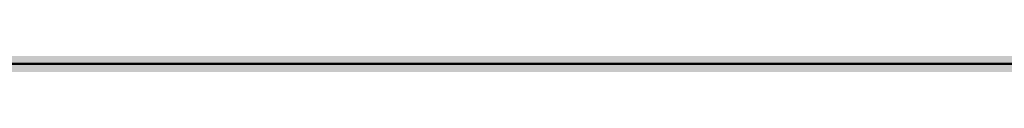
# Model space of a CAD drawing. Units: millimetres. Extents: x 0 to 2267, y 0 to 1823.
# Tile 89 of 256: x 1600.369 to 1605.705, y 1227.247 to 1227.247. Entities that reach past the tile are written whole.
import ezdxf

# ---------------------------------------------------------------- set-up
doc = ezdxf.new("R2010")
doc.units = ezdxf.units.MM
doc.header["$MEASUREMENT"] = 0
doc.layers.add('M-HATC', color=252, linetype='Continuous', lineweight=18)
doc.layers.add('M-OUTL', color=7, linetype='Continuous', lineweight=50)

msp = doc.modelspace()

# ---------------------------------------------------------------- hatches: boundary and pattern name
at = {"layer": 'M-HATC'}
h = msp.add_hatch(color=256, dxfattribs=at)
h.dxf.hatch_style = 1
h.paths.add_polyline_path([(2055.771, 1603.062), (1381.0868, 1603.062), (1381.0868, 1598.062), (2055.771, 1598.062)])
h.paths.add_polyline_path([(2055.771, 1598.062), (1381.0868, 1598.062), (1381.0868, 1593.062), (2055.771, 1593.062)])
h.paths.add_polyline_path([(2051.3074, 1536.7609), (1385.5504, 1536.7609), (1385.5504, 1526.7609), (1387.5504, 1526.7609), (1388.5366, 1525.0528), (1385.3319, 1521.2335), (1385.3319, 1521.2226), (2050.2542, 1522.7491), (2048.3212, 1525.0528), (2049.3074, 1526.7609), (2051.3074, 1526.7609)])
edge = h.paths.add_edge_path()
edge.add_arc((1847.5345, 1379.1492), 135, 222.603061, 222.890851, ccw=False)
edge.add_line((1748.1663, 1287.7656), (1683.0921, 1287.7656))
edge.add_arc((1583.7239, 1379.1492), 135, 317.109149, 317.396939, ccw=False)
edge.add_arc((1678.9686, 1290.6707), 5, 222.8909, 317.1091, ccw=False)
edge.add_arc((1774.2133, 1379.1492), 135, 222.603061, 222.890851, ccw=False)
edge.add_line((1674.8451, 1287.7656), (1609.7709, 1287.7656))
edge.add_arc((1510.4027, 1379.1492), 135, 317.109149, 317.396939, ccw=False)
edge.add_arc((1605.6474, 1290.6707), 5, 222.8909, 317.1091, ccw=False)
edge.add_arc((1700.8921, 1379.1492), 135, 222.603061, 222.890851, ccw=False)
edge.add_line((1601.5239, 1287.7656), (1536.4497, 1287.7656))
edge.add_arc((1437.0815, 1379.1492), 135, 317.109149, 317.396939, ccw=False)
edge.add_arc((1532.3262, 1290.6707), 5, 222.8909, 317.1091, ccw=False)
edge.add_arc((1627.5709, 1379.1492), 135, 222.603061, 222.890851, ccw=False)
edge.add_line((1528.2027, 1287.7656), (1505.9289, 1287.7656))
edge.add_spline(control_points=[(1505.9289, 1287.7656), (1504.2622, 1287.7656), (1504.2622, 1282.7656), (1505.9289, 1282.7656)], knot_values=[0, 0, 0, 0, 5, 5, 5, 5], degree=3, periodic=0)
edge.add_line((1505.9289, 1282.7656), (1930.9289, 1282.7656))
edge.add_spline(control_points=[(1930.9289, 1282.7656), (1932.5956, 1282.7656), (1932.5956, 1287.7656), (1930.9289, 1287.7656)], knot_values=[0, 0, 0, 0, 5, 5, 5, 5], degree=3, periodic=0)
edge.add_line((1930.9289, 1287.7656), (1903.0557, 1287.7656))
edge.add_arc((1803.6875, 1379.1492), 135, 317.109149, 317.396939, ccw=False)
edge.add_arc((1898.9322, 1290.6707), 5, 222.8909, 317.1091, ccw=False)
edge.add_arc((1994.1769, 1379.1492), 135, 222.603061, 222.890851, ccw=False)
edge.add_line((1894.8087, 1287.7656), (1829.7345, 1287.7656))
edge.add_arc((1730.3663, 1379.1492), 135, 317.109149, 317.396939, ccw=False)
edge.add_arc((1825.611, 1290.6707), 5, 222.8909, 317.1091, ccw=False)
edge.add_arc((1920.8557, 1379.1492), 135, 222.603061, 222.890851, ccw=False)
edge.add_line((1821.4875, 1287.7656), (1756.4133, 1287.7656))
edge.add_arc((1657.0451, 1379.1492), 135, 317.109149, 317.396939, ccw=False)
edge.add_arc((1752.2898, 1290.6707), 5, 222.8909, 317.1091, ccw=False)
edge = h.paths.add_edge_path()
edge.add_spline(control_points=[(1843.4289, 1227.2475), (1845.0956, 1227.2475), (1845.0956, 1232.2475), (1843.4289, 1232.2475)], knot_values=[0, 0, 0, 0, 5, 5, 5, 5], degree=3, periodic=0)
edge.add_line((1843.4289, 1232.2475), (1593.4289, 1232.2475))
edge.add_spline(control_points=[(1593.4289, 1232.2475), (1591.7622, 1232.2475), (1591.7622, 1227.2475), (1593.4289, 1227.2475)], knot_values=[0, 0, 0, 0, 5, 5, 5, 5], degree=3, periodic=0)
edge.add_line((1593.4289, 1227.2475), (1843.4289, 1227.2475))
h.paths.add_polyline_path([(1905.9289, 1127.4171), (1530.9289, 1127.4171, 0.414214), (1520.9289, 1117.4171), (1530.9289, 1117.4171), (1915.9289, 1117.4171, 0.414214)])
edge = h.paths.add_edge_path()
edge.add_arc((1397.0858, 1498.4078), 12.7299, 90.78215, 190.87871, ccw=False)
edge.add_line((1396.912, 1511.1365), (1428.0097, 1511.3488))
edge.add_line((1428.0097, 1511.3488), (1433.0097, 1511.3488))
edge.add_line((1433.0097, 1511.3488), (1434.439, 1511.3488))
edge.add_arc((1419.474, 1498.0804), 20, 41.561, 74.08211)
edge.add_line((1424.9592, 1517.3135), (1399.9351, 1517.2561))
edge.add_spline(control_points=[(1399.9307, 1517.2561), (1399.884, 1517.2131), (1399.8328, 1517.1689), (1399.7774, 1517.1236)], knot_values=[11.567499, 11.567499, 11.567499, 11.567499, 11.814249, 11.814249, 11.814249, 11.814249], degree=3, periodic=0)
edge.add_spline(control_points=[(1399.6328, 1517.0099), (1399.5831, 1516.9721), (1399.5307, 1516.9338), (1399.4759, 1516.8947)], knot_values=[11.167718, 11.167718, 11.167718, 11.167718, 11.365188, 11.365188, 11.365188, 11.365188], degree=3, periodic=0)
edge.add_spline(control_points=[(1399.3398, 1516.8001), (1399.1514, 1516.6719), (1398.9384, 1516.5377), (1398.704, 1516.3994)], knot_values=[10.376405, 10.376405, 10.376405, 10.376405, 11.00994, 11.00994, 11.00994, 11.00994], degree=3, periodic=0)
edge.add_spline(control_points=[(1398.6572, 1516.3719), (1398.5789, 1516.326), (1398.4983, 1516.2797), (1398.4155, 1516.2331)], knot_values=[10.125175, 10.125175, 10.125175, 10.125175, 10.334406, 10.334406, 10.334406, 10.334406], degree=3, periodic=0)
edge.add_spline(control_points=[(1398.2642, 1516.1487), (1398.196, 1516.1111), (1398.1263, 1516.0732), (1398.0555, 1516.0351)], knot_values=[9.832246, 9.832246, 9.832246, 9.832246, 9.999658, 9.999658, 9.999658, 9.999658], degree=3, periodic=0)
edge.add_spline(control_points=[(1397.9987, 1516.0048), (1397.7312, 1515.8621), (1397.446, 1515.7171), (1397.1466, 1515.5714)], knot_values=[9.161808, 9.161808, 9.161808, 9.161808, 9.787769, 9.787769, 9.787769, 9.787769], degree=3, periodic=0)
edge.add_spline(control_points=[(1397.1466, 1515.5714), (1396.8418, 1515.423), (1396.5222, 1515.274), (1396.1914, 1515.1262)], knot_values=[8.524455, 8.524455, 8.524455, 8.524455, 9.161808, 9.161808, 9.161808, 9.161808], degree=3, periodic=0)
edge.add_spline(control_points=[(1396.0777, 1515.0756), (1395.9854, 1515.0348), (1395.8922, 1514.994), (1395.7983, 1514.9534)], knot_values=[8.275193, 8.275193, 8.275193, 8.275193, 8.451726, 8.451726, 8.451726, 8.451726], degree=3, periodic=0)
edge.add_spline(control_points=[(1395.6018, 1514.8691), (1395.4997, 1514.8257), (1395.3968, 1514.7824), (1395.2932, 1514.7394)], knot_values=[7.962917, 7.962917, 7.962917, 7.962917, 8.152764, 8.152764, 8.152764, 8.152764], degree=3, periodic=0)
edge.add_spline(control_points=[(1395.2116, 1514.7057), (1394.8278, 1514.5475), (1394.4345, 1514.3929), (1394.0364, 1514.2442)], knot_values=[7.21254, 7.21254, 7.21254, 7.21254, 7.913148, 7.913148, 7.913148, 7.913148], degree=3, periodic=0)
edge.add_spline(control_points=[(1394.0364, 1514.2442), (1393.7076, 1514.1214), (1393.3754, 1514.0027), (1393.0427, 1513.8895)], knot_values=[6.633733, 6.633733, 6.633733, 6.633733, 7.21254, 7.21254, 7.21254, 7.21254], degree=3, periodic=0)
edge.add_spline(control_points=[(1392.8214, 1513.815), (1392.7198, 1513.7812), (1392.6181, 1513.7479), (1392.5166, 1513.7152)], knot_values=[6.328796, 6.328796, 6.328796, 6.328796, 6.505493, 6.505493, 6.505493, 6.505493], degree=3, periodic=0)
edge.add_spline(control_points=[(1392.5166, 1513.7152), (1392.3187, 1513.6515), (1392.1212, 1513.59), (1391.9244, 1513.531)], knot_values=[5.984605, 5.984605, 5.984605, 5.984605, 6.328796, 6.328796, 6.328796, 6.328796], degree=3, periodic=0)
edge.add_spline(control_points=[(1391.7915, 1513.4915), (1391.3122, 1513.3501), (1390.8384, 1513.2239), (1390.3784, 1513.1171)], knot_values=[5.066697, 5.066697, 5.066697, 5.066697, 5.907055, 5.907055, 5.907055, 5.907055], degree=3, periodic=0)
edge.add_spline(control_points=[(1390.3784, 1513.1171), (1390.1797, 1513.071), (1389.9836, 1513.0284), (1389.7907, 1512.9899)], knot_values=[4.70367, 4.70367, 4.70367, 4.70367, 5.066695, 5.066695, 5.066695, 5.066695], degree=3, periodic=0)
edge.add_spline(control_points=[(1389.422, 1512.9204), (1389.2459, 1512.8892), (1389.0729, 1512.8617), (1388.9036, 1512.8381)], knot_values=[4.130571, 4.130571, 4.130571, 4.130571, 4.469816, 4.469816, 4.469816, 4.469816], degree=3, periodic=0)
edge.add_spline(control_points=[(1388.9036, 1512.8381), (1388.591, 1512.7946), (1388.2911, 1512.7644), (1388.0071, 1512.7494)], knot_values=[3.504031, 3.504031, 3.504031, 3.504031, 4.130571, 4.130571, 4.130571, 4.130571], degree=3, periodic=0)
edge.add_spline(control_points=[(1387.9356, 1512.7459), (1387.8538, 1512.7423), (1387.7733, 1512.74), (1387.6944, 1512.739)], knot_values=[3.268866, 3.268866, 3.268866, 3.268866, 3.451164, 3.451164, 3.451164, 3.451164], degree=3, periodic=0)
edge.add_spline(control_points=[(1387.3351, 1512.7443), (1387.2076, 1512.7499), (1387.0847, 1512.7597), (1386.967, 1512.7739)], knot_values=[2.670686, 2.670686, 2.670686, 2.670686, 2.984, 2.984, 2.984, 2.984], degree=3, periodic=0)
edge.add_spline(control_points=[(1386.8327, 1512.7922), (1386.8209, 1512.7941), (1386.8092, 1512.7959), (1386.7975, 1512.7979)], knot_values=[2.516981, 2.516981, 2.516981, 2.516981, 2.549528, 2.549528, 2.549528, 2.549528], degree=3, periodic=0)
edge.add_spline(control_points=[(1386.4526, 1512.8735), (1386.4257, 1512.881), (1386.3993, 1512.889), (1386.3733, 1512.8972)], knot_values=[2.095869, 2.095869, 2.095869, 2.095869, 2.17941, 2.17941, 2.17941, 2.17941], degree=3, periodic=0)
edge.add_spline(control_points=[(1386.0691, 1513.0189), (1386.0634, 1513.0217), (1386.0577, 1513.0246), (1386.052, 1513.0275)], knot_values=[1.72453, 1.72453, 1.72453, 1.72453, 1.745933, 1.745933, 1.745933, 1.745933], degree=3, periodic=0)
edge.add_arc((1399.474, 1498.0804), 20, 131.82432, 180)
edge.add_arc((1630.3336, 1505.5484), 250.9708, 181.705176, 236.427975)
edge.add_arc((1605.3399, 1483.3044), 218.7822, 238.660829, 243.34961)
edge.add_arc((1647.0911, 1510.3592), 262.8986, 183.129836, 237.853442, ccw=False)
h.paths.add_polyline_path([(1406.5369, 1391.9644, 0.149382), (1491.5506, 1296.4418, -0.129517)], flags=17)
edge = h.paths.add_edge_path()
edge.add_arc((2037.3838, 1498.0804), 20, 0, 48.26587)
edge.add_spline(control_points=[(2050.6973, 1513.0052), (2050.6512, 1512.9847), (2050.6034, 1512.9655), (2050.5539, 1512.9477)], knot_values=[1.835652, 1.835652, 1.835652, 1.835652, 2.000781, 2.000781, 2.000781, 2.000781], degree=3, periodic=0)
edge.add_spline(control_points=[(2050.4616, 1512.9166), (2050.479, 1512.9221), (2050.4963, 1512.9277), (2050.5133, 1512.9335)], knot_values=[2.045477, 2.045477, 2.045477, 2.045477, 2.101389, 2.101389, 2.101389, 2.101389], degree=3, periodic=0)
edge.add_spline(control_points=[(2050.129, 1512.8342), (2050.1984, 1512.8473), (2050.2657, 1512.8623), (2050.3308, 1512.8792)], knot_values=[2.237629, 2.237629, 2.237629, 2.237629, 2.435841, 2.435841, 2.435841, 2.435841], degree=3, periodic=0)
edge.add_spline(control_points=[(2050.0946, 1512.8278), (2050.1061, 1512.8299), (2050.1176, 1512.832), (2050.129, 1512.8342)], knot_values=[2.435841, 2.435841, 2.435841, 2.435841, 2.468321, 2.468321, 2.468321, 2.468321], degree=3, periodic=0)
edge.add_spline(control_points=[(2049.7843, 1512.7851), (2049.8552, 1512.7922), (2049.9243, 1512.8008), (2049.9917, 1512.8109)], knot_values=[2.563852, 2.563852, 2.563852, 2.563852, 2.748541, 2.748541, 2.748541, 2.748541], degree=3, periodic=0)
edge.add_spline(control_points=[(2049.4052, 1512.7617), (2049.5364, 1512.7653), (2049.6629, 1512.773), (2049.7843, 1512.7851)], knot_values=[2.748541, 2.748541, 2.748541, 2.748541, 3.064882, 3.064882, 3.064882, 3.064882], degree=3, periodic=0)
edge.add_spline(control_points=[(2049.1698, 1512.7597), (2049.2336, 1512.7591), (2049.2965, 1512.7594), (2049.3584, 1512.7606)], knot_values=[3.102309, 3.102309, 3.102309, 3.102309, 3.2503, 3.2503, 3.2503, 3.2503], degree=3, periodic=0)
edge.add_spline(control_points=[(2048.8573, 1512.7691), (2048.9638, 1512.7638), (2049.068, 1512.7606), (2049.1698, 1512.7597)], knot_values=[3.2503, 3.2503, 3.2503, 3.2503, 3.486069, 3.486069, 3.486069, 3.486069], degree=3, periodic=0)
edge.add_spline(control_points=[(2048.6924, 1512.7789), (2048.3729, 1512.8009), (2048.0345, 1512.8411), (2047.6817, 1512.897)], knot_values=[3.606429, 3.606429, 3.606429, 3.606429, 4.2989, 4.2989, 4.2989, 4.2989], degree=3, periodic=0)
edge.add_spline(control_points=[(2047.6817, 1512.897), (2047.5458, 1512.9185), (2047.4077, 1512.9424), (2047.2678, 1512.9685)], knot_values=[4.2989, 4.2989, 4.2989, 4.2989, 4.565769, 4.565769, 4.565769, 4.565769], degree=3, periodic=0)
edge.add_spline(control_points=[(2047.2678, 1512.9685), (2047.1449, 1512.9914), (2047.0207, 1513.016), (2046.8951, 1513.0422)], knot_values=[4.565769, 4.565769, 4.565769, 4.565769, 4.799971, 4.799971, 4.799971, 4.799971], degree=3, periodic=0)
edge.add_spline(control_points=[(2046.8951, 1513.0422), (2046.5286, 1513.1188), (2046.1513, 1513.209), (2045.7676, 1513.3107)], knot_values=[4.799971, 4.799971, 4.799971, 4.799971, 5.483718, 5.483718, 5.483718, 5.483718], degree=3, periodic=0)
edge.add_spline(control_points=[(2045.7676, 1513.3107), (2045.3724, 1513.4154), (2044.9704, 1513.5322), (2044.5662, 1513.6588)], knot_values=[5.483718, 5.483718, 5.483718, 5.483718, 6.187866, 6.187866, 6.187866, 6.187866], degree=3, periodic=0)
edge.add_spline(control_points=[(2044.5662, 1513.6588), (2044.4149, 1513.7061), (2044.2633, 1513.7549), (2044.1116, 1513.8048)], knot_values=[6.187866, 6.187866, 6.187866, 6.187866, 6.451551, 6.451551, 6.451551, 6.451551], degree=3, periodic=0)
edge.add_spline(control_points=[(2044.1116, 1513.8048), (2043.9967, 1513.8427), (2043.8817, 1513.8813), (2043.7668, 1513.9205)], knot_values=[6.451551, 6.451551, 6.451551, 6.451551, 6.651434, 6.651434, 6.651434, 6.651434], degree=3, periodic=0)
edge.add_spline(control_points=[(2043.7668, 1513.9205), (2043.3716, 1514.0554), (2042.9774, 1514.1979), (2042.5886, 1514.3458)], knot_values=[6.651434, 6.651434, 6.651434, 6.651434, 7.338879, 7.338879, 7.338879, 7.338879], degree=3, periodic=0)
edge.add_spline(control_points=[(2042.5886, 1514.3458), (2042.1643, 1514.5071), (2041.7465, 1514.6749), (2041.3409, 1514.846)], knot_values=[7.338879, 7.338879, 7.338879, 7.338879, 8.089209, 8.089209, 8.089209, 8.089209], degree=3, periodic=0)
edge.add_spline(control_points=[(2041.3409, 1514.846), (2041.1028, 1514.9465), (2040.869, 1515.0481), (2040.6405, 1515.1502)], knot_values=[8.089209, 8.089209, 8.089209, 8.089209, 8.529587, 8.529587, 8.529587, 8.529587], degree=3, periodic=0)
edge.add_spline(control_points=[(2040.51, 1515.2089), (2040.0824, 1515.4022), (2039.6747, 1515.5971), (2039.295, 1515.7894)], knot_values=[8.613818, 8.613818, 8.613818, 8.613818, 9.44571, 9.44571, 9.44571, 9.44571], degree=3, periodic=0)
edge.add_spline(control_points=[(2039.295, 1515.7894), (2039.0618, 1515.9075), (2038.8391, 1516.0246), (2038.6288, 1516.1398)], knot_values=[9.44571, 9.44571, 9.44571, 9.44571, 9.956404, 9.956404, 9.956404, 9.956404], degree=3, periodic=0)
edge.add_spline(control_points=[(2038.6288, 1516.1398), (2038.5187, 1516.2001), (2038.4121, 1516.2598), (2038.309, 1516.3189)], knot_values=[9.956404, 9.956404, 9.956404, 9.956404, 10.223542, 10.223542, 10.223542, 10.223542], degree=3, periodic=0)
edge.add_spline(control_points=[(2038.309, 1516.3189), (2038.2138, 1516.3735), (2038.1216, 1516.4276), (2038.0328, 1516.481)], knot_values=[10.223542, 10.223542, 10.223542, 10.223542, 10.47051, 10.47051, 10.47051, 10.47051], degree=3, periodic=0)
edge.add_spline(control_points=[(2038.0328, 1516.481), (2037.7855, 1516.6296), (2037.5639, 1516.773), (2037.3722, 1516.909)], knot_values=[10.47051, 10.47051, 10.47051, 10.47051, 11.15767, 11.15767, 11.15767, 11.15767], degree=3, periodic=0)
edge.add_spline(control_points=[(2037.3722, 1516.909), (2037.2789, 1516.9752), (2037.1927, 1517.0396), (2037.1142, 1517.102)], knot_values=[11.15767, 11.15767, 11.15767, 11.15767, 11.49227, 11.49227, 11.49227, 11.49227], degree=3, periodic=0)
edge.add_spline(control_points=[(2036.8564, 1517.3259), (2036.9148, 1517.2692), (2036.9814, 1517.2103), (2037.0557, 1517.1492)], knot_values=[11.577341, 11.577341, 11.577341, 11.577341, 11.91035, 11.91035, 11.91035, 11.91035], degree=3, periodic=0)
edge.add_spline(control_points=[(2036.8074, 1517.3748), (2036.823, 1517.3587), (2036.8393, 1517.3424), (2036.8564, 1517.3259)], knot_values=[11.91035, 11.91035, 11.91035, 11.91035, 12.007402, 12.007402, 12.007402, 12.007402], degree=3, periodic=0)
edge.add_spline(control_points=[(2036.7017, 1517.494), (2036.7104, 1517.483), (2036.7196, 1517.4719), (2036.7291, 1517.4606)], knot_values=[12.184155, 12.184155, 12.184155, 12.184155, 12.255409, 12.255409, 12.255409, 12.255409], degree=3, periodic=0)
edge.add_spline(control_points=[(2036.6159, 1517.6205), (2036.62, 1517.613), (2036.6243, 1517.6055), (2036.6289, 1517.5979)], knot_values=[12.487913, 12.487913, 12.487913, 12.487913, 12.541035, 12.541035, 12.541035, 12.541035], degree=3, periodic=0)
edge.add_spline(control_points=[(2036.5635, 1517.786), (2036.5637, 1517.7794), (2036.5642, 1517.7726), (2036.565, 1517.7658)], knot_values=[12.911761, 12.911761, 12.911761, 12.911761, 12.968286, 12.968286, 12.968286, 12.968286], degree=3, periodic=0)
edge.add_spline(control_points=[(2036.6166, 1517.9304), (2036.6125, 1517.9259), (2036.6086, 1517.9212), (2036.6049, 1517.9165)], knot_values=[13.382527, 13.382527, 13.382527, 13.382527, 13.433791, 13.433791, 13.433791, 13.433791], degree=3, periodic=0)
edge.add_spline(control_points=[(2036.749, 1518.017), (2036.7361, 1518.0116), (2036.7239, 1518.006), (2036.7124, 1518.0002)], knot_values=[13.726299, 13.726299, 13.726299, 13.726299, 13.809928, 13.809928, 13.809928, 13.809928], degree=3, periodic=0)
edge.add_spline(control_points=[(2036.8604, 1518.0528), (2036.8386, 1518.0474), (2036.8181, 1518.0416), (2036.7988, 1518.0353)], knot_values=[13.910887, 13.910887, 13.910887, 13.910887, 14.02153, 14.02153, 14.02153, 14.02153], degree=3, periodic=0)
edge.add_line((2036.9639, 1518.0804), (2032.3838, 1518.0804))
edge.add_line((2032.3838, 1518.0804), (2027.3838, 1518.0804))
edge.add_line((2027.3838, 1518.0804), (2022.3838, 1518.0804))
edge.add_line((2022.3838, 1518.0804), (2017.3838, 1518.0804))
edge.add_arc((2017.3838, 1498.0804), 20, 90, 138.439)
edge.add_line((2002.4188, 1511.3488), (2003.8481, 1511.3488))
edge.add_line((2003.8481, 1511.3488), (2008.8481, 1511.3488))
edge.add_line((2008.8481, 1511.3488), (2039.772, 1511.1377))
edge.add_arc((2039.772, 1498.4078), 12.7299, -10.87871, 90, ccw=False)
edge.add_arc((1789.7668, 1510.3592), 262.8986, 302.146558, 356.870164, ccw=False)
edge.add_arc((1831.5179, 1483.3044), 218.7822, 296.65039, 301.339171)
edge.add_arc((1806.5242, 1505.5484), 250.9708, 303.572025, 358.294824)
h.paths.add_polyline_path([(2030.321, 1391.9644, -0.129517), (1945.3072, 1296.4418, 0.149382)], flags=17)
edge = h.paths.add_edge_path()
edge.add_spline(control_points=[(2037.2464, 1518.0821), (2037.2898, 1518.081), (2037.3355, 1518.0804), (2037.3838, 1518.0804)], knot_values=[0.000012, 0.000012, 0.000012, 0.000012, 0.144754, 0.144754, 0.144754, 0.144754], degree=3, periodic=0)
edge.add_line((2037.3357, 1518.0804), (2037.0096, 1518.0804))
edge.add_spline(control_points=[(2037.0096, 1518.0804), (2036.9822, 1518.0768), (2036.956, 1518.0727), (2036.9312, 1518.0681)], knot_values=[14.13465, 14.13465, 14.13465, 14.13465, 14.247197, 14.247197, 14.247197, 14.247197], degree=3, periodic=0)
edge.add_spline(control_points=[(2036.9312, 1518.0681), (2036.9276, 1518.0674), (2036.9241, 1518.0667), (2036.9205, 1518.0661)], knot_values=[14.118315, 14.118315, 14.118315, 14.118315, 14.13465, 14.13465, 14.13465, 14.13465], degree=3, periodic=0)
edge.add_spline(control_points=[(2036.9205, 1518.0661), (2036.9118, 1518.0644), (2036.9032, 1518.0626), (2036.8948, 1518.0608)], knot_values=[14.078086, 14.078086, 14.078086, 14.078086, 14.118315, 14.118315, 14.118315, 14.118315], degree=3, periodic=0)
edge.add_spline(control_points=[(2036.8948, 1518.0608), (2036.883, 1518.0583), (2036.8716, 1518.0556), (2036.8604, 1518.0528)], knot_values=[14.02153, 14.02153, 14.02153, 14.02153, 14.078086, 14.078086, 14.078086, 14.078086], degree=3, periodic=0)
edge.add_spline(control_points=[(2036.8604, 1518.0528), (2036.8386, 1518.0474), (2036.8181, 1518.0416), (2036.7988, 1518.0353)], knot_values=[13.910887, 13.910887, 13.910887, 13.910887, 14.02153, 14.02153, 14.02153, 14.02153], degree=3, periodic=0)
edge.add_spline(control_points=[(2036.7988, 1518.0353), (2036.7981, 1518.035), (2036.7974, 1518.0348), (2036.7967, 1518.0346)], knot_values=[13.906906, 13.906906, 13.906906, 13.906906, 13.910887, 13.910887, 13.910887, 13.910887], degree=3, periodic=0)
edge.add_spline(control_points=[(2036.7967, 1518.0346), (2036.7882, 1518.0318), (2036.7799, 1518.0289), (2036.7719, 1518.0259)], knot_values=[13.857826, 13.857826, 13.857826, 13.857826, 13.906906, 13.906906, 13.906906, 13.906906], degree=3, periodic=0)
edge.add_spline(control_points=[(2036.7719, 1518.0259), (2036.764, 1518.023), (2036.7564, 1518.02), (2036.749, 1518.017)], knot_values=[13.809928, 13.809928, 13.809928, 13.809928, 13.857826, 13.857826, 13.857826, 13.857826], degree=3, periodic=0)
edge.add_spline(control_points=[(2036.749, 1518.017), (2036.7361, 1518.0116), (2036.7239, 1518.006), (2036.7124, 1518.0002)], knot_values=[13.726299, 13.726299, 13.726299, 13.726299, 13.809928, 13.809928, 13.809928, 13.809928], degree=3, periodic=0)
edge.add_spline(control_points=[(2036.7124, 1518.0002), (2036.7121, 1518), (2036.7118, 1517.9999), (2036.7115, 1517.9997)], knot_values=[13.723993, 13.723993, 13.723993, 13.723993, 13.726299, 13.726299, 13.726299, 13.726299], degree=3, periodic=0)
edge.add_spline(control_points=[(2036.7115, 1517.9997), (2036.7063, 1517.9971), (2036.7013, 1517.9944), (2036.6965, 1517.9917)], knot_values=[13.686536, 13.686536, 13.686536, 13.686536, 13.723993, 13.723993, 13.723993, 13.723993], degree=3, periodic=0)
edge.add_spline(control_points=[(2036.6965, 1517.9917), (2036.6919, 1517.9891), (2036.6874, 1517.9865), (2036.6831, 1517.9839)], knot_values=[13.651251, 13.651251, 13.651251, 13.651251, 13.686536, 13.686536, 13.686536, 13.686536], degree=3, periodic=0)
edge.add_spline(control_points=[(2036.6831, 1517.9839), (2036.6764, 1517.9798), (2036.67, 1517.9757), (2036.6639, 1517.9714)], knot_values=[13.596804, 13.596804, 13.596804, 13.596804, 13.651251, 13.651251, 13.651251, 13.651251], degree=3, periodic=0)
edge.add_spline(control_points=[(2036.6639, 1517.9714), (2036.6636, 1517.9712), (2036.6633, 1517.9709), (2036.6629, 1517.9707)], knot_values=[13.593956, 13.593956, 13.593956, 13.593956, 13.596804, 13.596804, 13.596804, 13.596804], degree=3, periodic=0)
edge.add_spline(control_points=[(2036.6629, 1517.9707), (2036.6603, 1517.9689), (2036.6577, 1517.967), (2036.6552, 1517.9651)], knot_values=[13.570322, 13.570322, 13.570322, 13.570322, 13.593956, 13.593956, 13.593956, 13.593956], degree=3, periodic=0)
edge.add_spline(control_points=[(2036.6552, 1517.9651), (2036.6525, 1517.9631), (2036.6499, 1517.9611), (2036.6474, 1517.9591)], knot_values=[13.545477, 13.545477, 13.545477, 13.545477, 13.570322, 13.570322, 13.570322, 13.570322], degree=3, periodic=0)
edge.add_spline(control_points=[(2036.6474, 1517.9591), (2036.6472, 1517.9589), (2036.6471, 1517.9588), (2036.6469, 1517.9587)], knot_values=[13.543931, 13.543931, 13.543931, 13.543931, 13.545477, 13.545477, 13.545477, 13.545477], degree=3, periodic=0)
edge.add_spline(control_points=[(2036.6469, 1517.9587), (2036.6412, 1517.9541), (2036.6358, 1517.9494), (2036.6307, 1517.9447)], knot_values=[13.488237, 13.488237, 13.488237, 13.488237, 13.543931, 13.543931, 13.543931, 13.543931], degree=3, periodic=0)
edge.add_spline(control_points=[(2036.6307, 1517.9447), (2036.6282, 1517.9423), (2036.6257, 1517.9399), (2036.6233, 1517.9374)], knot_values=[13.460307, 13.460307, 13.460307, 13.460307, 13.488237, 13.488237, 13.488237, 13.488237], degree=3, periodic=0)
edge.add_spline(control_points=[(2036.6233, 1517.9374), (2036.6215, 1517.9356), (2036.6198, 1517.9338), (2036.6181, 1517.932)], knot_values=[13.439712, 13.439712, 13.439712, 13.439712, 13.460307, 13.460307, 13.460307, 13.460307], degree=3, periodic=0)
edge.add_spline(control_points=[(2036.6181, 1517.932), (2036.6176, 1517.9315), (2036.6171, 1517.9309), (2036.6166, 1517.9304)], knot_values=[13.433791, 13.433791, 13.433791, 13.433791, 13.439712, 13.439712, 13.439712, 13.439712], degree=3, periodic=0)
edge.add_spline(control_points=[(2036.6166, 1517.9304), (2036.6125, 1517.9259), (2036.6086, 1517.9212), (2036.6049, 1517.9165)], knot_values=[13.382527, 13.382527, 13.382527, 13.382527, 13.433791, 13.433791, 13.433791, 13.433791], degree=3, periodic=0)
edge.add_spline(control_points=[(2036.6049, 1517.9165), (2036.6026, 1517.9135), (2036.6004, 1517.9104), (2036.5982, 1517.9074)], knot_values=[13.350017, 13.350017, 13.350017, 13.350017, 13.382527, 13.382527, 13.382527, 13.382527], degree=3, periodic=0)
edge.add_spline(control_points=[(2036.5982, 1517.9074), (2036.5972, 1517.9059), (2036.5962, 1517.9043), (2036.5952, 1517.9028)], knot_values=[13.333922, 13.333922, 13.333922, 13.333922, 13.350017, 13.350017, 13.350017, 13.350017], degree=3, periodic=0)
edge.add_spline(control_points=[(2036.5952, 1517.9028), (2036.5945, 1517.9018), (2036.5939, 1517.9009), (2036.5933, 1517.8999)], knot_values=[13.323828, 13.323828, 13.323828, 13.323828, 13.333922, 13.333922, 13.333922, 13.333922], degree=3, periodic=0)
edge.add_spline(control_points=[(2036.5933, 1517.8999), (2036.5905, 1517.8955), (2036.5879, 1517.8909), (2036.5855, 1517.8864)], knot_values=[13.277545, 13.277545, 13.277545, 13.277545, 13.323828, 13.323828, 13.323828, 13.323828], degree=3, periodic=0)
edge.add_spline(control_points=[(2036.5855, 1517.8864), (2036.5836, 1517.8827), (2036.5817, 1517.8789), (2036.5801, 1517.8751)], knot_values=[13.240119, 13.240119, 13.240119, 13.240119, 13.277545, 13.277545, 13.277545, 13.277545], degree=3, periodic=0)
edge.add_spline(control_points=[(2036.5801, 1517.8751), (2036.5795, 1517.8739), (2036.579, 1517.8727), (2036.5785, 1517.8715)], knot_values=[13.228211, 13.228211, 13.228211, 13.228211, 13.240119, 13.240119, 13.240119, 13.240119], degree=3, periodic=0)
edge.add_spline(control_points=[(2036.5785, 1517.8715), (2036.578, 1517.8702), (2036.5774, 1517.869), (2036.5769, 1517.8677)], knot_values=[13.215717, 13.215717, 13.215717, 13.215717, 13.228211, 13.228211, 13.228211, 13.228211], degree=3, periodic=0)
edge.add_spline(control_points=[(2036.5769, 1517.8677), (2036.5755, 1517.864), (2036.5741, 1517.8603), (2036.5729, 1517.8565)], knot_values=[13.179847, 13.179847, 13.179847, 13.179847, 13.215717, 13.215717, 13.215717, 13.215717], degree=3, periodic=0)
edge.add_spline(control_points=[(2036.5729, 1517.8565), (2036.5713, 1517.8515), (2036.5699, 1517.8464), (2036.5687, 1517.8413)], knot_values=[13.132017, 13.132017, 13.132017, 13.132017, 13.179847, 13.179847, 13.179847, 13.179847], degree=3, periodic=0)
edge.add_spline(control_points=[(2036.5687, 1517.8413), (2036.5684, 1517.8402), (2036.5682, 1517.8392), (2036.568, 1517.8382)], knot_values=[13.122482, 13.122482, 13.122482, 13.122482, 13.132017, 13.132017, 13.132017, 13.132017], degree=3, periodic=0)
edge.add_spline(control_points=[(2036.568, 1517.8382), (2036.5676, 1517.8363), (2036.5672, 1517.8345), (2036.5669, 1517.8327)], knot_values=[13.105592, 13.105592, 13.105592, 13.105592, 13.122482, 13.122482, 13.122482, 13.122482], degree=3, periodic=0)
edge.add_spline(control_points=[(2036.5669, 1517.8327), (2036.5662, 1517.8292), (2036.5657, 1517.8257), (2036.5652, 1517.8222)], knot_values=[13.074063, 13.074063, 13.074063, 13.074063, 13.105592, 13.105592, 13.105592, 13.105592], degree=3, periodic=0)
edge.add_spline(control_points=[(2036.5652, 1517.8222), (2036.5652, 1517.8222), (2036.5652, 1517.8222), (2036.5652, 1517.8222)], knot_values=[13.074043, 13.074043, 13.074043, 13.074043, 13.074063, 13.074063, 13.074063, 13.074063], degree=3, periodic=0)
edge.add_spline(control_points=[(2036.5652, 1517.8222), (2036.5644, 1517.8164), (2036.5639, 1517.8106), (2036.5636, 1517.8046)], knot_values=[13.021884, 13.021884, 13.021884, 13.021884, 13.074043, 13.074043, 13.074043, 13.074043], degree=3, periodic=0)
edge.add_spline(control_points=[(2036.5636, 1517.8046), (2036.5636, 1517.804), (2036.5636, 1517.8034), (2036.5635, 1517.8028)], knot_values=[13.01674, 13.01674, 13.01674, 13.01674, 13.021884, 13.021884, 13.021884, 13.021884], degree=3, periodic=0)
edge.add_spline(control_points=[(2036.5635, 1517.8028), (2036.5634, 1517.8005), (2036.5634, 1517.7982), (2036.5634, 1517.7958)], knot_values=[12.996438, 12.996438, 12.996438, 12.996438, 13.01674, 13.01674, 13.01674, 13.01674], degree=3, periodic=0)
edge.add_spline(control_points=[(2036.5634, 1517.7958), (2036.5633, 1517.7926), (2036.5634, 1517.7893), (2036.5635, 1517.786)], knot_values=[12.968286, 12.968286, 12.968286, 12.968286, 12.996438, 12.996438, 12.996438, 12.996438], degree=3, periodic=0)
edge.add_spline(control_points=[(2036.5635, 1517.786), (2036.5637, 1517.7794), (2036.5642, 1517.7726), (2036.565, 1517.7658)], knot_values=[12.911761, 12.911761, 12.911761, 12.911761, 12.968286, 12.968286, 12.968286, 12.968286], degree=3, periodic=0)
edge.add_spline(control_points=[(2036.565, 1517.7658), (2036.565, 1517.7657), (2036.565, 1517.7656), (2036.565, 1517.7656)], knot_values=[12.911017, 12.911017, 12.911017, 12.911017, 12.911761, 12.911761, 12.911761, 12.911761], degree=3, periodic=0)
edge.add_spline(control_points=[(2036.565, 1517.7656), (2036.5654, 1517.7625), (2036.5658, 1517.7593), (2036.5663, 1517.7562)], knot_values=[12.88528, 12.88528, 12.88528, 12.88528, 12.911017, 12.911017, 12.911017, 12.911017], degree=3, periodic=0)
edge.add_spline(control_points=[(2036.5663, 1517.7562), (2036.5667, 1517.7534), (2036.5672, 1517.7506), (2036.5677, 1517.7478)], knot_values=[12.862519, 12.862519, 12.862519, 12.862519, 12.88528, 12.88528, 12.88528, 12.88528], degree=3, periodic=0)
edge.add_spline(control_points=[(2036.5677, 1517.7478), (2036.5678, 1517.7474), (2036.5679, 1517.7469), (2036.568, 1517.7465)], knot_values=[12.858885, 12.858885, 12.858885, 12.858885, 12.862519, 12.862519, 12.862519, 12.862519], degree=3, periodic=0)
edge.add_spline(control_points=[(2036.568, 1517.7465), (2036.5692, 1517.7399), (2036.5707, 1517.7332), (2036.5724, 1517.7264)], knot_values=[12.8053, 12.8053, 12.8053, 12.8053, 12.858885, 12.858885, 12.858885, 12.858885], degree=3, periodic=0)
edge.add_spline(control_points=[(2036.5724, 1517.7264), (2036.5734, 1517.7226), (2036.5745, 1517.7187), (2036.5756, 1517.7149)], knot_values=[12.775176, 12.775176, 12.775176, 12.775176, 12.8053, 12.8053, 12.8053, 12.8053], degree=3, periodic=0)
edge.add_spline(control_points=[(2036.5756, 1517.7149), (2036.5763, 1517.7125), (2036.577, 1517.7102), (2036.5778, 1517.7078)], knot_values=[12.756759, 12.756759, 12.756759, 12.756759, 12.775176, 12.775176, 12.775176, 12.775176], degree=3, periodic=0)
edge.add_spline(control_points=[(2036.5778, 1517.7078), (2036.5781, 1517.7067), (2036.5784, 1517.7057), (2036.5787, 1517.7047)], knot_values=[12.748742, 12.748742, 12.748742, 12.748742, 12.756759, 12.756759, 12.756759, 12.756759], degree=3, periodic=0)
edge.add_spline(control_points=[(2036.5787, 1517.7047), (2036.5808, 1517.6983), (2036.5831, 1517.6919), (2036.5856, 1517.6854)], knot_values=[12.69959, 12.69959, 12.69959, 12.69959, 12.748742, 12.748742, 12.748742, 12.748742], degree=3, periodic=0)
edge.add_spline(control_points=[(2036.5856, 1517.6854), (2036.5876, 1517.68), (2036.5898, 1517.6746), (2036.5921, 1517.6692)], knot_values=[12.659038, 12.659038, 12.659038, 12.659038, 12.69959, 12.69959, 12.69959, 12.69959], degree=3, periodic=0)
edge.add_spline(control_points=[(2036.5921, 1517.6692), (2036.594, 1517.6648), (2036.5959, 1517.6605), (2036.5979, 1517.6561)], knot_values=[12.626806, 12.626806, 12.626806, 12.626806, 12.659038, 12.659038, 12.659038, 12.659038], degree=3, periodic=0)
edge.add_spline(control_points=[(2036.5979, 1517.6561), (2036.5984, 1517.6551), (2036.5989, 1517.6541), (2036.5993, 1517.6531)], knot_values=[12.619394, 12.619394, 12.619394, 12.619394, 12.626806, 12.626806, 12.626806, 12.626806], degree=3, periodic=0)
edge.add_spline(control_points=[(2036.5993, 1517.6531), (2036.6043, 1517.6424), (2036.6099, 1517.6315), (2036.6159, 1517.6205)], knot_values=[12.541039, 12.541039, 12.541039, 12.541039, 12.619394, 12.619394, 12.619394, 12.619394], degree=3, periodic=0)
edge.add_spline(control_points=[(2036.6159, 1517.6205), (2036.6159, 1517.6205), (2036.6159, 1517.6205), (2036.6159, 1517.6205)], knot_values=[12.541035, 12.541035, 12.541035, 12.541035, 12.541039, 12.541039, 12.541039, 12.541039], degree=3, periodic=0)
edge.add_spline(control_points=[(2036.6159, 1517.6205), (2036.62, 1517.613), (2036.6243, 1517.6055), (2036.6289, 1517.5979)], knot_values=[12.487913, 12.487913, 12.487913, 12.487913, 12.541035, 12.541035, 12.541035, 12.541035], degree=3, periodic=0)
edge.add_spline(control_points=[(2036.6289, 1517.5979), (2036.6326, 1517.5916), (2036.6365, 1517.5853), (2036.6406, 1517.5789)], knot_values=[12.443982, 12.443982, 12.443982, 12.443982, 12.487913, 12.487913, 12.487913, 12.487913], degree=3, periodic=0)
edge.add_spline(control_points=[(2036.6406, 1517.5789), (2036.6414, 1517.5776), (2036.6423, 1517.5763), (2036.6431, 1517.5749)], knot_values=[12.434996, 12.434996, 12.434996, 12.434996, 12.443982, 12.443982, 12.443982, 12.443982], degree=3, periodic=0)
edge.add_spline(control_points=[(2036.6431, 1517.5749), (2036.6531, 1517.5596), (2036.6639, 1517.5439), (2036.6756, 1517.528)], knot_values=[12.329647, 12.329647, 12.329647, 12.329647, 12.434996, 12.434996, 12.434996, 12.434996], degree=3, periodic=0)
edge.add_spline(control_points=[(2036.6756, 1517.528), (2036.6839, 1517.5168), (2036.6925, 1517.5055), (2036.7017, 1517.494)], knot_values=[12.255409, 12.255409, 12.255409, 12.255409, 12.329647, 12.329647, 12.329647, 12.329647], degree=3, periodic=0)
edge.add_spline(control_points=[(2036.7017, 1517.494), (2036.7104, 1517.483), (2036.7196, 1517.4719), (2036.7291, 1517.4606)], knot_values=[12.184155, 12.184155, 12.184155, 12.184155, 12.255409, 12.255409, 12.255409, 12.255409], degree=3, periodic=0)
edge.add_spline(control_points=[(2036.7291, 1517.4606), (2036.7436, 1517.4435), (2036.759, 1517.4262), (2036.7753, 1517.4085)], knot_values=[12.075961, 12.075961, 12.075961, 12.075961, 12.184155, 12.184155, 12.184155, 12.184155], degree=3, periodic=0)
edge.add_spline(control_points=[(2036.7753, 1517.4085), (2036.7763, 1517.4075), (2036.7773, 1517.4064), (2036.7783, 1517.4054)], knot_values=[12.069502, 12.069502, 12.069502, 12.069502, 12.075961, 12.075961, 12.075961, 12.075961], degree=3, periodic=0)
edge.add_spline(control_points=[(2036.7783, 1517.4054), (2036.7877, 1517.3953), (2036.7974, 1517.385), (2036.8074, 1517.3748)], knot_values=[12.007402, 12.007402, 12.007402, 12.007402, 12.069502, 12.069502, 12.069502, 12.069502], degree=3, periodic=0)
edge.add_spline(control_points=[(2036.8074, 1517.3748), (2036.823, 1517.3587), (2036.8393, 1517.3424), (2036.8564, 1517.3259)], knot_values=[11.91035, 11.91035, 11.91035, 11.91035, 12.007402, 12.007402, 12.007402, 12.007402], degree=3, periodic=0)
edge.add_spline(control_points=[(2036.8564, 1517.3259), (2036.9148, 1517.2692), (2036.9814, 1517.2103), (2037.0557, 1517.1492)], knot_values=[11.577341, 11.577341, 11.577341, 11.577341, 11.91035, 11.91035, 11.91035, 11.91035], degree=3, periodic=0)
edge.add_spline(control_points=[(2037.0557, 1517.1492), (2037.0747, 1517.1336), (2037.0942, 1517.1179), (2037.1142, 1517.102)], knot_values=[11.49227, 11.49227, 11.49227, 11.49227, 11.577341, 11.577341, 11.577341, 11.577341], degree=3, periodic=0)
edge.add_spline(control_points=[(2037.1142, 1517.102), (2037.1927, 1517.0396), (2037.2789, 1516.9752), (2037.3722, 1516.909)], knot_values=[11.15767, 11.15767, 11.15767, 11.15767, 11.49227, 11.49227, 11.49227, 11.49227], degree=3, periodic=0)
edge.add_spline(control_points=[(2037.3722, 1516.909), (2037.5639, 1516.773), (2037.7855, 1516.6296), (2038.0328, 1516.481)], knot_values=[10.47051, 10.47051, 10.47051, 10.47051, 11.15767, 11.15767, 11.15767, 11.15767], degree=3, periodic=0)
edge.add_spline(control_points=[(2038.0328, 1516.481), (2038.1216, 1516.4276), (2038.2138, 1516.3735), (2038.309, 1516.3189)], knot_values=[10.223542, 10.223542, 10.223542, 10.223542, 10.47051, 10.47051, 10.47051, 10.47051], degree=3, periodic=0)
edge.add_spline(control_points=[(2038.309, 1516.3189), (2038.4121, 1516.2598), (2038.5187, 1516.2001), (2038.6288, 1516.1398)], knot_values=[9.956404, 9.956404, 9.956404, 9.956404, 10.223542, 10.223542, 10.223542, 10.223542], degree=3, periodic=0)
edge.add_spline(control_points=[(2038.6288, 1516.1398), (2038.8391, 1516.0246), (2039.0618, 1515.9075), (2039.295, 1515.7894)], knot_values=[9.44571, 9.44571, 9.44571, 9.44571, 9.956404, 9.956404, 9.956404, 9.956404], degree=3, periodic=0)
edge.add_spline(control_points=[(2039.295, 1515.7894), (2039.6747, 1515.5971), (2040.0824, 1515.4022), (2040.51, 1515.2089)], knot_values=[8.613818, 8.613818, 8.613818, 8.613818, 9.44571, 9.44571, 9.44571, 9.44571], degree=3, periodic=0)
edge.add_spline(control_points=[(2040.51, 1515.2089), (2040.5533, 1515.1893), (2040.5968, 1515.1697), (2040.6405, 1515.1502)], knot_values=[8.529587, 8.529587, 8.529587, 8.529587, 8.613818, 8.613818, 8.613818, 8.613818], degree=3, periodic=0)
edge.add_spline(control_points=[(2040.6405, 1515.1502), (2040.869, 1515.0481), (2041.1028, 1514.9465), (2041.3409, 1514.846)], knot_values=[8.089209, 8.089209, 8.089209, 8.089209, 8.529587, 8.529587, 8.529587, 8.529587], degree=3, periodic=0)
edge.add_spline(control_points=[(2041.3409, 1514.846), (2041.7465, 1514.6749), (2042.1643, 1514.5071), (2042.5886, 1514.3458)], knot_values=[7.338879, 7.338879, 7.338879, 7.338879, 8.089209, 8.089209, 8.089209, 8.089209], degree=3, periodic=0)
edge.add_spline(control_points=[(2042.5886, 1514.3458), (2042.9774, 1514.1979), (2043.3716, 1514.0554), (2043.7668, 1513.9205)], knot_values=[6.651434, 6.651434, 6.651434, 6.651434, 7.338879, 7.338879, 7.338879, 7.338879], degree=3, periodic=0)
edge.add_spline(control_points=[(2043.7668, 1513.9205), (2043.8817, 1513.8813), (2043.9967, 1513.8427), (2044.1116, 1513.8048)], knot_values=[6.451551, 6.451551, 6.451551, 6.451551, 6.651434, 6.651434, 6.651434, 6.651434], degree=3, periodic=0)
edge.add_spline(control_points=[(2044.1116, 1513.8048), (2044.2633, 1513.7549), (2044.4149, 1513.7061), (2044.5662, 1513.6588)], knot_values=[6.187866, 6.187866, 6.187866, 6.187866, 6.451551, 6.451551, 6.451551, 6.451551], degree=3, periodic=0)
edge.add_spline(control_points=[(2044.5662, 1513.6588), (2044.9704, 1513.5322), (2045.3724, 1513.4154), (2045.7676, 1513.3107)], knot_values=[5.483718, 5.483718, 5.483718, 5.483718, 6.187866, 6.187866, 6.187866, 6.187866], degree=3, periodic=0)
edge.add_spline(control_points=[(2045.7676, 1513.3107), (2046.1513, 1513.209), (2046.5286, 1513.1188), (2046.8951, 1513.0422)], knot_values=[4.799971, 4.799971, 4.799971, 4.799971, 5.483718, 5.483718, 5.483718, 5.483718], degree=3, periodic=0)
edge.add_spline(control_points=[(2046.8951, 1513.0422), (2047.0207, 1513.016), (2047.1449, 1512.9914), (2047.2678, 1512.9685)], knot_values=[4.565769, 4.565769, 4.565769, 4.565769, 4.799971, 4.799971, 4.799971, 4.799971], degree=3, periodic=0)
edge.add_spline(control_points=[(2047.2678, 1512.9685), (2047.4077, 1512.9424), (2047.5458, 1512.9185), (2047.6817, 1512.897)], knot_values=[4.2989, 4.2989, 4.2989, 4.2989, 4.565769, 4.565769, 4.565769, 4.565769], degree=3, periodic=0)
edge.add_spline(control_points=[(2047.6817, 1512.897), (2048.0345, 1512.8411), (2048.3729, 1512.8009), (2048.6924, 1512.7789)], knot_values=[3.606429, 3.606429, 3.606429, 3.606429, 4.2989, 4.2989, 4.2989, 4.2989], degree=3, periodic=0)
edge.add_spline(control_points=[(2048.6924, 1512.7789), (2048.7479, 1512.7751), (2048.8029, 1512.7718), (2048.8573, 1512.7691)], knot_values=[3.486069, 3.486069, 3.486069, 3.486069, 3.606429, 3.606429, 3.606429, 3.606429], degree=3, periodic=0)
edge.add_spline(control_points=[(2048.8573, 1512.7691), (2048.9638, 1512.7638), (2049.068, 1512.7606), (2049.1698, 1512.7597)], knot_values=[3.2503, 3.2503, 3.2503, 3.2503, 3.486069, 3.486069, 3.486069, 3.486069], degree=3, periodic=0)
edge.add_spline(control_points=[(2049.1698, 1512.7597), (2049.2336, 1512.7591), (2049.2965, 1512.7594), (2049.3584, 1512.7606)], knot_values=[3.102309, 3.102309, 3.102309, 3.102309, 3.2503, 3.2503, 3.2503, 3.2503], degree=3, periodic=0)
edge.add_spline(control_points=[(2049.3584, 1512.7606), (2049.3741, 1512.7609), (2049.3897, 1512.7613), (2049.4052, 1512.7617)], knot_values=[3.064882, 3.064882, 3.064882, 3.064882, 3.102309, 3.102309, 3.102309, 3.102309], degree=3, periodic=0)
edge.add_spline(control_points=[(2049.4052, 1512.7617), (2049.5364, 1512.7653), (2049.6629, 1512.773), (2049.7843, 1512.7851)], knot_values=[2.748541, 2.748541, 2.748541, 2.748541, 3.064882, 3.064882, 3.064882, 3.064882], degree=3, periodic=0)
edge.add_spline(control_points=[(2049.7843, 1512.7851), (2049.8552, 1512.7922), (2049.9243, 1512.8008), (2049.9917, 1512.8109)], knot_values=[2.563852, 2.563852, 2.563852, 2.563852, 2.748541, 2.748541, 2.748541, 2.748541], degree=3, periodic=0)
edge.add_spline(control_points=[(2049.9917, 1512.8109), (2050.0265, 1512.8161), (2050.0608, 1512.8218), (2050.0946, 1512.8278)], knot_values=[2.468321, 2.468321, 2.468321, 2.468321, 2.563852, 2.563852, 2.563852, 2.563852], degree=3, periodic=0)
edge.add_spline(control_points=[(2050.0946, 1512.8278), (2050.1061, 1512.8299), (2050.1176, 1512.832), (2050.129, 1512.8342)], knot_values=[2.435841, 2.435841, 2.435841, 2.435841, 2.468321, 2.468321, 2.468321, 2.468321], degree=3, periodic=0)
edge.add_spline(control_points=[(2050.129, 1512.8342), (2050.1984, 1512.8473), (2050.2657, 1512.8623), (2050.3308, 1512.8792)], knot_values=[2.237629, 2.237629, 2.237629, 2.237629, 2.435841, 2.435841, 2.435841, 2.435841], degree=3, periodic=0)
edge.add_spline(control_points=[(2050.3308, 1512.8792), (2050.3754, 1512.8908), (2050.4191, 1512.9032), (2050.4616, 1512.9166)], knot_values=[2.101389, 2.101389, 2.101389, 2.101389, 2.237629, 2.237629, 2.237629, 2.237629], degree=3, periodic=0)
edge.add_spline(control_points=[(2050.4616, 1512.9166), (2050.479, 1512.9221), (2050.4963, 1512.9277), (2050.5133, 1512.9335)], knot_values=[2.045477, 2.045477, 2.045477, 2.045477, 2.101389, 2.101389, 2.101389, 2.101389], degree=3, periodic=0)
edge.add_spline(control_points=[(2050.5133, 1512.9335), (2050.527, 1512.9382), (2050.5405, 1512.9429), (2050.5539, 1512.9477)], knot_values=[2.000781, 2.000781, 2.000781, 2.000781, 2.045477, 2.045477, 2.045477, 2.045477], degree=3, periodic=0)
edge.add_spline(control_points=[(2050.5539, 1512.9477), (2050.6034, 1512.9655), (2050.6512, 1512.9847), (2050.6973, 1513.0052)], knot_values=[1.835652, 1.835652, 1.835652, 1.835652, 2.000781, 2.000781, 2.000781, 2.000781], degree=3, periodic=0)
edge.add_arc((2037.3838, 1498.0804), 20, 48.26587, 90.12993)
edge = h.paths.add_edge_path(flags=16)
edge.add_spline(control_points=[(1386.1389, 1512.9859), (1388.92, 1511.7395), (1398.0387, 1515.5187), (1399.9307, 1517.2561)], knot_values=[1.831046, 1.831046, 1.831046, 1.831046, 11.814249, 11.814249, 11.814249, 11.814249], degree=3, periodic=0)
edge.add_line((1399.9307, 1517.2561), (1393.7435, 1517.2419))
edge.add_arc((1399.474, 1498.0804), 20, 106.6501, 131.8173)
h = msp.add_hatch(color=256, dxfattribs=at)
h.dxf.hatch_style = 1
h.paths.add_polyline_path([(2042.8886, 1580.1796), (2055.771, 1593.062), (1381.0868, 1593.062), (1393.9692, 1580.1796), (1374.086, 1560.2964), (2062.7718, 1560.2964)])
h.paths.add_polyline_path([(1843.4289, 1201.3297), (1843.4289, 1227.2475), (1593.4289, 1227.2475), (1593.4289, 1201.3297, -0.228274), (1574.5989, 1162.2346), (1530.9289, 1127.4171), (1905.9289, 1127.4171), (1862.2589, 1162.2346, -0.228274)])

# ---------------------------------------------------------------- linework, layer by layer
at = {"layer": 'M-OUTL'}
msp.add_line((1593.4289, 1227.2475), (1843.4289, 1227.2475), dxfattribs=at)

doc.saveas('drawing.dxf')
